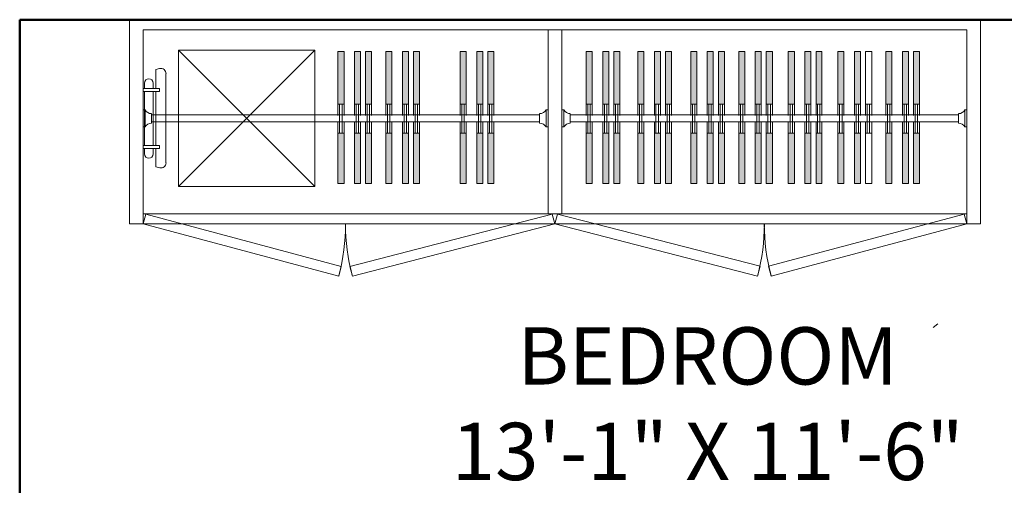
# Model space of a CAD drawing. Units: inches. Extents: x -466983 to 1020, y 324 to 318697.
# Tile 4 of 97: x 452 to 555, y 514 to 563. Entities that reach past the tile are written whole.
import ezdxf

# ---------------------------------------------------------------- set-up
doc = ezdxf.new("R2010")
doc.units = ezdxf.units.IN
doc.header["$MEASUREMENT"] = 0
for name, color, linetype, lineweight in [('A-AREA-IDEN', 7, 'Continuous', 25), ('A-FURN', 8, 'Continuous', 18), ('A-WALL', 7, 'Continuous', 50)]:
    doc.layers.add(name, color=color, linetype=linetype, lineweight=lineweight)
doc.styles.get("Standard").update_dxf_attribs({"font": 'arial.ttf'})

# ---------------------------------------------------------------- blocks, each defined once
blk = doc.blocks.new('A$C05F852CF')
for p, q in [((0.0306, 3.0783), (0.4692, 3.0783)), ((0.4692, 3.0783), (2.0768, 3.0783)), ((0.52, 3.0783), (0.52, 1.0783)), ((2.02, 3.0783), (2.02, 1.0783)), ((2.0768, 3.0783), (2.5066, 3.0783)), ((0, 3.0548), (0, 2.6659)), ((0.5, 3.0423), (0.5, 2.6496)), ((2.04, 3.05), (2.04, 2.6642)), ((0.52, 3.0283), (2.02, 3.0283)), ((2.54, 2.6547), (2.54, 3.0393)), ((0.2418, 2.9702), (0.2418, 3.0002)), ((0.5609, 3.0045), (0.5953, 2.9829)), ((0.5609, 3.0045), (0.6121, 2.9725)), ((1.2427, 2.9995), (1.1927, 2.9682)), ((2.2982, 2.9702), (2.2982, 3.0002)), ((0.6121, 2.9725), (0.6546, 2.9682)), ((1.1927, 2.9682), (1.1672, 2.9661)), ((0.1349, 2.8634), (0.1049, 2.8634)), ((0.3487, 2.8634), (0.3787, 2.8634)), ((2.1913, 2.8634), (2.1613, 2.8634)), ((2.4051, 2.8634), (2.4351, 2.8634)), ((0.2418, 2.7265), (0.2418, 2.7565)), ((2.2982, 2.7265), (2.2982, 2.7565)), ((0.5711, 2.6712), (0.6015, 2.7135)), ((0.6015, 2.7135), (0.6164, 2.7178)), ((1.1864, 2.7072), (1.1588, 2.7242)), ((1.2397, 2.6852), (1.1864, 2.7072)), ((1.0379, 2.6608), (0.52, 2.2697)), ((2.02, 2.6608), (1.0379, 2.6608)), ((1.7737, 2.6608), (1.7737, 1.0783)), ((1.7937, 2.6608), (1.7937, 1.0783)), ((1.8137, 2.6608), (1.8137, 1.0783)), ((1.8337, 2.6608), (1.8337, 1.0783)), ((0.0322, 2.6283), (0.4826, 2.6283)), ((2.0707, 2.6283), (2.5056, 2.6283)), ((0.52, 1.4597), (2.02, 1.4597)), ((0.52, 1.4397), (2.02, 1.4397)), ((0.52, 1.4197), (2.02, 1.4197)), ((0.52, 1.3997), (2.02, 1.3997)), ((0.52, 1.0783), (2.02, 1.0783)), ((0.726, 0.4346), (0.7377, 0.4444))]:
    blk.add_line(p, q)
for points in [[(1.3405, 2.9829), (1.306, 3.0045), (1.3573, 2.9725), (1.3998, 2.9682)], [(1.9879, 2.9995), (1.9379, 2.9682), (1.9124, 2.9661)], [(1.3162, 2.6712), (1.3467, 2.7135), (1.3616, 2.7178)], [(1.9848, 2.6852), (1.9315, 2.7072), (1.9039, 2.7242)]]:
    blk.add_lwpolyline(points)
for points in [[(1.0353, 2.1379, -0.173032), (1.022, 2.6388), (0.536, 2.2719, 0.053888)], [(1.7081, 1.7759, 0.101392), (1.7282, 1.7501, -0.223768), (1.7345, 1.736, -0.25558), (1.7315, 1.7308, -0.081563), (1.7151, 1.724, -0.071805), (1.6967, 1.7225, 0.069985), (1.6778, 1.7209, 0.03546), (1.6148, 1.7021, 0.029432), (1.5425, 1.6697, 0.001554), (1.5078, 1.6515, -0.00152), (1.4724, 1.6329, -0.004735), (1.4356, 1.6142, 0.00382), (1.3901, 1.5911, 0.296001), (1.3692, 1.5546, -0.649774), (1.3468, 1.5431, -0.02319), (1.3416, 1.5477, 0.0288), (1.3374, 1.5514, 0.005727), (1.3298, 1.557, -0.004358), (1.3198, 1.5645, -0.027528), (1.3001, 1.5812, -0.046214), (1.29, 1.5928, -0.194121), (1.2856, 1.6105, 0.133719), (1.2823, 1.6363, 0.011505), (1.2622, 1.682, 0.008882), (1.2338, 1.7401, 0.012426), (1.1937, 1.8139, -0.033612), (1.1801, 1.8418), (1.1552, 1.9026), (1.1361, 1.9495, 0.224341), (1.1204, 1.9638, -0.722772), (1.1202, 1.9734, -0.103513), (1.1242, 1.9739, 0.053465), (1.132, 1.9742, 0.030109), (1.1569, 1.9792, -0.031436), (1.1808, 1.984, -0.05324), (1.1971, 1.9844, 0.05518), (1.2128, 1.9849, 0.056271), (1.2402, 1.992, 0.0108), (1.3759, 2.0475, 0.00456), (1.4675, 2.0883, 0.01125), (1.5041, 2.106, 0.069394), (1.5235, 2.1196, -0.079756), (1.5405, 2.1311, -0.106399), (1.5562, 2.1345, -0.328642), (1.5608, 2.1312, -0.299547), (1.5587, 2.124, 0.189917), (1.5536, 2.1141, 0.033518), (1.5531, 2.1029, 0.075627), (1.554, 2.0981, 0.053489), (1.5579, 2.0898, 0.017838), (1.5727, 2.0672, 0.038394), (1.5932, 2.0425, -0.059529), (1.6058, 2.026, -0.035943), (1.6193, 1.9987, -0.011245), (1.6541, 1.9079, -0.006203), (1.6684, 1.8661, 0.010783), (1.6769, 1.8422, 0.019485), (1.6828, 1.8283, 0.005062)], [(1.6953, 1.7695, 0.098587), (1.7181, 1.7399, -0.040378), (1.7118, 1.7379, -0.071805), (1.6975, 1.7367, 0.069985), (1.6747, 1.7349, 0.03546), (1.6097, 1.7154, 0.029432), (1.5359, 1.6824, 0.001554), (1.5012, 1.6641, -0.00152), (1.4658, 1.6456, -0.004735), (1.4293, 1.627, 0.00382), (1.3835, 1.6038, 0.289814), (1.3549, 1.555, -0.018279), (1.3515, 1.5579, 0.0288), (1.3461, 1.5627, 0.005727), (1.3382, 1.5686, -0.004358), (1.3285, 1.5758, -0.027528), (1.31, 1.5916, -0.046214), (1.3016, 1.6012, -0.194121), (1.2997, 1.6085, 0.133719), (1.2955, 1.6417, 0.011505), (1.2752, 1.6881, 0.008882), (1.2465, 1.7466, 0.012426), (1.2061, 1.821, -0.033612), (1.1933, 1.8472), (1.1684, 1.908), (1.1493, 1.9549, 0.051417), (1.1455, 1.962, 0.017208), (1.1606, 1.9654, -0.031436), (1.1827, 1.9698, -0.05324), (1.196, 1.9702, 0.05518), (1.2149, 1.9708, 0.056271), (1.2453, 1.9787, 0.0108), (1.3816, 2.0344, 0.00456), (1.4734, 2.0753, 0.01125), (1.5106, 2.0933, 0.069394), (1.5332, 2.1091, -0.038161), (1.5392, 2.114, 0.029361), (1.5389, 2.1025, 0.075627), (1.5405, 2.0934, 0.053489), (1.5457, 2.0824, 0.017838), (1.5611, 2.0589, 0.038394), (1.583, 2.0326, -0.059529), (1.5935, 2.0187, -0.035943), (1.6061, 1.9933, -0.011245), (1.6406, 1.9031, -0.006203), (1.6549, 1.8617, 0.010783), (1.6635, 1.8371, 0.019485), (1.6699, 1.8222, 0.005062)]]:
    blk.add_lwpolyline(points, format="xyb", close=True)
for points in [[(1.27, 1.665, 0.025626), (1.2575, 1.662, 0.0108), (1.1179, 1.617, 0.00456), (1.0234, 1.5834, 0.01125), (0.9856, 1.5685, 0.069394), (0.9653, 1.5565, -0.079756), (0.9474, 1.5464, -0.106399), (0.9315, 1.5441, -0.328642), (0.9272, 1.5478, -0.299547), (0.9298, 1.5548, 0.189917), (0.9357, 1.5643, 0.033518), (0.9369, 1.5754, 0.075627), (0.9364, 1.5803, 0.053489), (0.9332, 1.5888, 0.017838), (0.9202, 1.6125, 0.038394), (0.9016, 1.6387, -0.059529), (0.8903, 1.6561, -0.035943), (0.8789, 1.6844, -0.011245), (0.8512, 1.7776, -0.006203), (0.8402, 1.8203, 0.010783), (0.8336, 1.8448, 0.019485), (0.8287, 1.8592, 0.005062), (0.8076, 1.9133, 0.101392), (0.7895, 1.9406, -0.223768), (0.7843, 1.9551, -0.25558), (0.7876, 1.9601, -0.081563), (0.8046, 1.9656, -0.071805), (0.823, 1.9657, 0.069985), (0.842, 1.9658, 0.03546), (0.9062, 1.9798, 0.029432), (0.9807, 2.0065, 0.001554), (1.0167, 2.022, -0.00152), (1.0535, 2.0378, -0.004735), (1.0916, 2.0536, 0.00382), (1.1388, 2.0731, 0.296001), (1.1624, 2.108, -0.649774), (1.1856, 2.1178, -0.02319), (1.1904, 2.1128, 0.0288), (1.1944, 2.1088, 0.005727), (1.2015, 2.1025, -0.004358), (1.2108, 2.0944, -0.027528), (1.2292, 2.0762, -0.046214), (1.2384, 2.0638, -0.194121), (1.2414, 2.0458, 0.133719), (1.2427, 2.0199, 0.005779), (1.2507, 1.9961)], [(1.2674, 1.6787, 0.025626), (1.2535, 1.6753, 0.0108), (1.1134, 1.6301, 0.00456), (1.0187, 1.5964, 0.01125), (0.9802, 1.5813, 0.069394), (0.9566, 1.5673, -0.042175), (0.9495, 1.5626, 0.031457), (0.9508, 1.5747, 0.075627), (0.9499, 1.5838, 0.053489), (0.9456, 1.595, 0.017838), (0.9321, 1.6196, 0.038394), (0.9123, 1.6476, -0.059529), (0.9028, 1.6622, -0.035943), (0.8922, 1.6886, -0.011245), (0.8646, 1.7812, -0.006203), (0.8536, 1.8236, 0.010783), (0.8469, 1.8487, 0.019485), (0.8417, 1.8641, 0.005062), (0.8204, 1.9185, 0.100237), (0.7996, 1.9501, -0.044209), (0.8066, 1.9519, -0.071805), (0.8211, 1.952, 0.069985), (0.8439, 1.9521, 0.03546), (0.9101, 1.9665, 0.029432), (0.9862, 1.9937, 0.001554), (1.0222, 2.0093, -0.00152), (1.0589, 2.025, -0.004735), (1.0968, 2.0408, 0.00382), (1.1442, 2.0604, 0.294287), (1.1763, 2.1074, -0.02184), (1.18, 2.1036, 0.0288), (1.1851, 2.0984, 0.005727), (1.1924, 2.092, -0.004358), (1.2016, 2.084, -0.027528), (1.2189, 2.0669, -0.046214), (1.2266, 2.0566, -0.194121), (1.2279, 2.0488, 0.133719), (1.2295, 2.0156, 0.005779), (1.2376, 1.9915, 0.005779)]]:
    blk.add_lwpolyline(points, format="xyb")
for centre, radius in [((0.2418, 2.8634), 0.1369), ((2.2982, 2.8634), 0.1369), ((0.2418, 2.8634), 0.1069), ((2.2982, 2.8634), 0.1069)]:
    blk.add_circle(centre, radius)
for centre, radius, start, end in [((1.7308, 2.407), 0.7379, 159.8846, 202.2194), ((1.4058, 4.5145), 2.4132, 248.4641, 261.4655)]:
    blk.add_arc(centre, radius, start, end)
for points in [[(0, 3.0548), (0, 3.0677), (0.0177, 3.0783), (0.0306, 3.0783)], [(0.5, 3.0423), (0.5, 3.0581), (0.485, 3.0783), (0.4692, 3.0783)], [(2.04, 3.05), (2.04, 3.0655), (2.0613, 3.0783), (2.0768, 3.0783)], [(2.5066, 3.0783), (2.5237, 3.0783), (2.54, 3.0564), (2.54, 3.0393)], [(0.0322, 2.6283), (0.0157, 2.6283), (0, 2.6494), (0, 2.6659)], [(2.04, 2.6642), (2.04, 2.6485), (2.055, 2.6283), (2.0707, 2.6283)], [(2.5056, 2.6283), (2.5201, 2.6283), (2.54, 2.6403), (2.54, 2.6547)], [(0.5, 2.6496), (0.5, 2.6405), (0.4918, 2.6283), (0.4826, 2.6283)]]:
    blk.add_open_spline(points, degree=3)
for points, knots in [([(0.5609, 3.0045), (0.565, 2.9818), (0.5836, 2.9366), (0.5776, 2.889), (0.5689, 2.8351), (0.5832, 2.7709), (0.5808, 2.7088), (0.5744, 2.6927), (0.5693, 2.6651), (0.5803, 2.6793), (0.5989, 2.6876), (0.7172, 2.6598), (0.8681, 2.7029), (1.0484, 2.6781), (1.0324, 2.6731), (1.1431, 2.7116), (1.202, 2.6757), (1.2459, 2.6867), (1.2222, 2.695), (1.2359, 2.7251), (1.2468, 2.781), (1.2288, 2.8492), (1.2515, 2.925), (1.2279, 2.9609), (1.2471, 3.0058), (1.2098, 2.9902), (1.1177, 3.0095), (0.956, 3.0159), (0.9532, 2.9758), (0.7999, 3.021), (0.7569, 3.0151), (0.5986, 2.9869), (0.561, 3.0049)], [16.816032, 16.816032, 16.816032, 16.816032, 79.038845, 88.513895, 147.565266, 227.196862, 259.685448, 283.955301, 296.511304, 302.432558, 320.230942, 354.322559, 575.279549, 734.72356, 845.740421, 943.033103, 1029.533967, 1032.845074, 1043.313584, 1065.311534, 1104.921835, 1208.53002, 1248.510714, 1303.102727, 1321.01326, 1329.647833, 1389.371624, 1571.817644, 1750.274161, 1823.189073, 1967.937033, 2020.912329, 2020.912329, 2020.912329, 2020.912329]), ([(1.306, 3.0045), (1.3102, 2.9818), (1.3287, 2.9366), (1.3228, 2.889), (1.314, 2.8351), (1.3284, 2.7709), (1.3259, 2.7088), (1.3196, 2.6927), (1.3144, 2.6651), (1.3254, 2.6793), (1.3441, 2.6876), (1.4624, 2.6598), (1.6132, 2.7029), (1.6436, 2.6781), (1.7775, 2.6731), (1.8882, 2.7116), (1.9472, 2.6757), (1.9911, 2.6867), (1.9673, 2.695), (1.981, 2.7251), (1.992, 2.781), (1.974, 2.8492), (1.9967, 2.925), (1.9731, 2.9609), (1.9922, 3.0058), (1.9549, 2.9902), (1.8628, 3.0095), (1.7011, 3.0159), (1.5483, 2.9758), (1.5451, 3.021), (1.5021, 3.0151), (1.3437, 2.9869), (1.3062, 3.0049)], [16.816032, 16.816032, 16.816032, 16.816032, 79.038845, 88.513895, 147.565266, 227.196862, 259.685448, 283.955301, 296.511304, 302.432558, 320.230942, 354.322559, 575.279549, 734.72356, 845.740421, 943.033103, 1029.533967, 1032.845074, 1043.313584, 1065.311534, 1104.921835, 1208.53002, 1248.510714, 1303.102727, 1321.01326, 1329.647833, 1389.371624, 1571.817644, 1750.274161, 1823.189073, 1967.937033, 2020.912329, 2020.912329, 2020.912329, 2020.912329]), ([(1.186, 2.943), (1.1557, 2.9456), (1.1387, 2.9502), (1.0976, 2.9551), (1.0776, 2.9567), (1.0342, 2.9582), (1.0123, 2.957), (0.991, 2.9533), (0.9902, 2.9517), (0.962, 2.9403), (0.9371, 2.935), (0.8851, 2.9413), (0.8522, 2.9513), (0.8033, 2.9629), (0.7938, 2.964), (0.755, 2.9608), (0.7319, 2.9572), (0.6794, 2.9481), (0.658, 2.9434), (0.631, 2.9418)], [1364.380335, 1364.380335, 1364.380335, 1364.380335, 1423.60231, 1423.60231, 1482.824284, 1482.824284, 1566.205036, 1566.205036, 1649.585789, 1649.585789, 1732.966542, 1732.966542, 1816.347295, 1816.347295, 1899.728048, 1899.728048, 1960.499853, 1960.499853, 1990.525565, 1990.525565, 1990.525565, 1990.525565]), ([(0.631, 2.9418), (0.6332, 2.9288), (0.633, 2.9104), (0.6308, 2.893), (0.6298, 2.8865), (0.628, 2.8726), (0.6273, 2.866), (0.6257, 2.8474), (0.6257, 2.8375), (0.629, 2.8013), (0.6345, 2.7696), (0.6337, 2.7333)], [67.285362, 67.285362, 67.285362, 67.285362, 87.399558, 87.399558, 107.513754, 107.513754, 127.62795, 127.62795, 167.856341, 167.856341, 238.127268, 238.127268, 238.127268, 238.127268]), ([(1.1845, 2.7412), (1.189, 2.7552), (1.1894, 2.765), (1.1874, 2.7998), (1.1843, 2.8219), (1.1844, 2.8664), (1.1882, 2.8901), (1.192, 2.9105), (1.1922, 2.9144), (1.1921, 2.9158), (1.1908, 2.9212), (1.1875, 2.9351), (1.1867, 2.9388), (1.186, 2.943)], [1072.516901, 1072.516901, 1072.516901, 1072.516901, 1129.100964, 1129.100964, 1185.685027, 1185.685027, 1226.035089, 1226.035089, 1249.281274, 1249.281274, 1272.52746, 1272.52746, 1279.689275, 1279.689275, 1279.689275, 1279.689275]), ([(1.3759, 2.942), (1.3781, 2.929), (1.378, 2.9106), (1.3757, 2.893), (1.3748, 2.8866), (1.373, 2.8727), (1.3722, 2.8661), (1.3706, 2.8475), (1.3707, 2.8375), (1.3739, 2.8012), (1.3795, 2.7694), (1.3787, 2.7331)], [67.156228, 67.156228, 67.156228, 67.156228, 87.297212, 87.297212, 107.438196, 107.438196, 127.57918, 127.57918, 167.861148, 167.861148, 238.25357, 238.25357, 238.25357, 238.25357]), ([(1.5104, 2.9621), (1.4964, 2.9606), (1.4732, 2.9568), (1.4226, 2.948), (1.4017, 2.9435), (1.3759, 2.942)], [1904.3965, 1904.3965, 1904.3965, 1904.3965, 1961.927876, 1961.927876, 1990.619445, 1990.619445, 1990.619445, 1990.619445]), ([(1.9314, 2.9432), (1.8997, 2.9459), (1.8822, 2.9507), (1.8387, 2.9557), (1.8168, 2.9572), (1.7515, 2.9587), (1.7088, 2.9551), (1.6403, 2.9447), (1.6154, 2.9402), (1.5795, 2.937), (1.5675, 2.9361), (1.5394, 2.9412), (1.5201, 2.9507), (1.5104, 2.9621)], [1364.265661, 1364.265661, 1364.265661, 1364.265661, 1426.240795, 1426.240795, 1488.215928, 1488.215928, 1612.166195, 1612.166195, 1689.92864, 1689.92864, 1733.064362, 1733.064362, 1768.978829, 1768.978829, 1768.978829, 1768.978829]), ([(1.9299, 2.7409), (1.9344, 2.755), (1.9348, 2.7648), (1.9328, 2.7996), (1.9297, 2.8217), (1.9298, 2.8662), (1.9336, 2.8899), (1.9374, 2.9105), (1.9376, 2.9144), (1.9375, 2.9159), (1.9362, 2.9214), (1.9329, 2.9353), (1.9321, 2.939), (1.9314, 2.9432)], [1072.238498, 1072.238498, 1072.238498, 1072.238498, 1128.864869, 1128.864869, 1185.491239, 1185.491239, 1225.989553, 1225.989553, 1249.326401, 1249.326401, 1272.66325, 1272.66325, 1279.788508, 1279.788508, 1279.788508, 1279.788508]), ([(0.6337, 2.7333), (0.6515, 2.7301), (0.6627, 2.7284), (0.6898, 2.7263), (0.7032, 2.726), (0.7436, 2.727), (0.7707, 2.73), (0.8409, 2.7383), (0.8881, 2.7432), (0.9755, 2.7406), (1.0125, 2.7357), (1.0356, 2.7309), (1.0369, 2.7307), (1.0381, 2.7304)], [345.4047, 345.4047, 345.4047, 345.4047, 383.386056, 383.386056, 421.367413, 421.367413, 497.330126, 497.330126, 611.561469, 611.561469, 725.792813, 725.792813, 732.434768, 732.434768, 732.434768, 732.434768]), ([(1.0381, 2.7304), (1.0497, 2.7345), (1.0742, 2.7435), (1.1251, 2.7504), (1.1528, 2.749), (1.1769, 2.7432), (1.1809, 2.7421), (1.1845, 2.7412)], [843.64503, 843.64503, 843.64503, 843.64503, 911.27572, 911.27572, 959.088062, 959.088062, 969.47998, 969.47998, 969.47998, 969.47998]), ([(1.3787, 2.7331), (1.3984, 2.7296), (1.4106, 2.7278), (1.4401, 2.7258), (1.4545, 2.7258), (1.4962, 2.7276), (1.5219, 2.7313), (1.5767, 2.7399), (1.6067, 2.7436), (1.6527, 2.7371), (1.662, 2.7326), (1.7084, 2.7282), (1.7364, 2.7276), (1.7849, 2.734), (1.8076, 2.7406), (1.8563, 2.7489), (1.8812, 2.7508), (1.914, 2.7451), (1.9226, 2.7428), (1.9299, 2.7409)], [345.267918, 345.267918, 345.267918, 345.267918, 387.167414, 387.167414, 429.06691, 429.06691, 512.865903, 512.865903, 629.317545, 629.317545, 745.769188, 745.769188, 834.622813, 834.622813, 901.414409, 901.414409, 948.921878, 948.921878, 969.679511, 969.679511, 969.679511, 969.679511])]:
    blk.add_open_spline(points, degree=3, knots=knots)
for p in [(0.2366, 2.8475), (2.3034, 2.8475), (0.2309, 2.8244), (2.02, 1.0783), (2.02, 1.0783)]:
    blk.add_point(p)
blk = doc.blocks.new('Wardrobe')
h = blk.add_hatch(color=256)
h.dxf.hatch_style = 1
h.paths.add_polyline_path([(2766.95, 1539.75), (2766.16, 1539.75), (2766.16, 1532.86), (2766.95, 1532.86)])
h.paths.add_polyline_path([(2766.95, 1529.07), (2766.16, 1529.07), (2766.16, 1522.48), (2766.95, 1522.48)])
h.paths.add_polyline_path([(2799.41, 1529.07), (2798.63, 1529.07), (2798.63, 1522.47), (2799.41, 1522.47)])
h.paths.add_polyline_path([(2799.41, 1539.75), (2798.63, 1539.75), (2798.63, 1532.86), (2799.41, 1532.86)])
h.paths.add_polyline_path([(2813.08, 1539.75), (2812.29, 1539.75), (2812.29, 1532.86), (2813.08, 1532.86)])
h.paths.add_polyline_path([(2813.08, 1529.07), (2812.29, 1529.07), (2812.29, 1522.47), (2813.08, 1522.47)])
h.paths.add_polyline_path([(2825.84, 1539.75), (2825.05, 1539.75), (2825.05, 1532.86), (2825.84, 1532.86)])
h.paths.add_polyline_path([(2825.84, 1529.07), (2825.05, 1529.07), (2825.05, 1522.47), (2825.84, 1522.47)])
h.paths.add_polyline_path([(2782.93, 1539.75), (2782.14, 1539.75), (2782.14, 1532.86), (2782.93, 1532.86)])
h.paths.add_polyline_path([(2782.93, 1529.07), (2782.14, 1529.07), (2782.14, 1522.48), (2782.93, 1522.48)])
h.paths.add_polyline_path([(2838.6, 1539.75), (2837.81, 1539.75), (2837.81, 1532.86), (2838.6, 1532.86)])
h.paths.add_polyline_path([(2838.6, 1529.07), (2837.81, 1529.07), (2837.81, 1522.47), (2838.6, 1522.47)])
h = blk.add_hatch(color=256)
h.dxf.hatch_style = 1
h.paths.add_polyline_path([(2769.11, 1539.75), (2768.32, 1539.75), (2768.32, 1532.86), (2769.11, 1532.86)])
h.paths.add_polyline_path([(2769.11, 1529.07), (2768.32, 1529.07), (2768.32, 1522.48), (2769.11, 1522.48)])
h.paths.add_polyline_path([(2801.57, 1539.75), (2800.79, 1539.75), (2800.79, 1532.86), (2801.57, 1532.86)])
h.paths.add_polyline_path([(2801.57, 1529.07), (2800.79, 1529.07), (2800.79, 1522.47), (2801.57, 1522.47)])
h.paths.add_polyline_path([(2815.24, 1539.75), (2814.45, 1539.75), (2814.45, 1532.86), (2815.24, 1532.86)])
h.paths.add_polyline_path([(2815.24, 1529.07), (2814.45, 1529.07), (2814.45, 1522.47), (2815.24, 1522.47)])
h.paths.add_polyline_path([(2828, 1529.07), (2827.21, 1529.07), (2827.21, 1522.47), (2828, 1522.47)])
h.paths.add_polyline_path([(2828, 1539.75), (2827.21, 1539.75), (2827.21, 1532.86), (2828, 1532.86)])
h.paths.add_polyline_path([(2840.76, 1539.75), (2839.97, 1539.75), (2839.97, 1532.86), (2840.76, 1532.86)])
h.paths.add_polyline_path([(2840.76, 1529.07), (2839.97, 1529.07), (2839.97, 1522.47), (2840.76, 1522.47)])
h.paths.add_polyline_path([(2785.09, 1539.75), (2784.3, 1539.75), (2784.3, 1532.86), (2785.09, 1532.86)])
h.paths.add_polyline_path([(2785.09, 1529.07), (2784.3, 1529.07), (2784.3, 1522.48), (2785.09, 1522.48)])
h = blk.add_hatch(color=256)
h.dxf.hatch_style = 1
h.paths.add_polyline_path([(2770.56, 1539.75), (2769.77, 1539.75), (2769.77, 1532.86), (2770.56, 1532.86)])
h.paths.add_polyline_path([(2770.56, 1529.07), (2769.77, 1529.07), (2769.77, 1522.48), (2770.56, 1522.48)])
h.paths.add_polyline_path([(2786.54, 1539.75), (2785.76, 1539.75), (2785.76, 1532.86), (2786.54, 1532.86)])
h.paths.add_polyline_path([(2786.54, 1529.07), (2785.76, 1529.07), (2785.76, 1522.48), (2786.54, 1522.48)])
h.paths.add_polyline_path([(2803.03, 1539.75), (2802.24, 1539.75), (2802.24, 1532.86), (2803.03, 1532.86)])
h.paths.add_polyline_path([(2803.03, 1529.07), (2802.24, 1529.07), (2802.24, 1522.47), (2803.03, 1522.47)])
h.paths.add_polyline_path([(2816.69, 1539.75), (2815.9, 1539.75), (2815.9, 1532.86), (2816.69, 1532.86)])
h.paths.add_polyline_path([(2816.69, 1529.07), (2815.9, 1529.07), (2815.9, 1522.47), (2816.69, 1522.47)])
h = blk.add_hatch(color=256)
h.dxf.hatch_style = 1
h.paths.add_polyline_path([(2773.22, 1539.75), (2772.43, 1539.75), (2772.43, 1532.86), (2773.22, 1532.86)])
h.paths.add_polyline_path([(2806.16, 1539.75), (2805.37, 1539.75), (2805.37, 1532.86), (2806.16, 1532.86)])
h.paths.add_polyline_path([(2806.16, 1529.07), (2805.37, 1529.07), (2805.37, 1522.47), (2806.16, 1522.47)])
h.paths.add_polyline_path([(2773.22, 1529.07), (2772.43, 1529.07), (2772.43, 1522.48), (2773.22, 1522.48)])
h.paths.add_polyline_path([(2819.35, 1539.75), (2818.56, 1539.75), (2818.56, 1532.86), (2819.35, 1532.86)])
h.paths.add_polyline_path([(2819.35, 1529.07), (2818.56, 1529.07), (2818.56, 1522.47), (2819.35, 1522.47)])
h.paths.add_polyline_path([(2832.33, 1539.75), (2831.54, 1539.75), (2831.54, 1532.86), (2832.33, 1532.86)])
h.paths.add_polyline_path([(2832.33, 1529.07), (2831.54, 1529.07), (2831.54, 1522.47), (2832.33, 1522.47)])
h = blk.add_hatch(color=256)
h.dxf.hatch_style = 1
h.paths.add_polyline_path([(2775.38, 1539.75), (2774.59, 1539.75), (2774.59, 1532.86), (2775.38, 1532.86)])
h.paths.add_polyline_path([(2775.38, 1529.07), (2774.59, 1529.07), (2774.59, 1522.48), (2775.38, 1522.48)])
h.paths.add_polyline_path([(2808.32, 1539.75), (2807.53, 1539.75), (2807.53, 1532.86), (2808.32, 1532.86)])
h.paths.add_polyline_path([(2808.32, 1529.07), (2807.53, 1529.07), (2807.53, 1522.47), (2808.32, 1522.47)])
h.paths.add_polyline_path([(2834.49, 1539.75), (2833.7, 1539.75), (2833.7, 1532.86), (2834.49, 1532.86)])
h.paths.add_polyline_path([(2834.49, 1529.07), (2833.7, 1529.07), (2833.7, 1522.47), (2834.49, 1522.47)])
h = blk.add_hatch(color=256)
h.dxf.hatch_style = 1
h.paths.add_polyline_path([(2776.83, 1539.75), (2776.04, 1539.75), (2776.04, 1532.86), (2776.83, 1532.86)])
h.paths.add_polyline_path([(2776.83, 1529.07), (2776.04, 1529.07), (2776.04, 1522.48), (2776.83, 1522.48)])
h.paths.add_polyline_path([(2809.77, 1539.75), (2808.98, 1539.75), (2808.98, 1532.86), (2809.77, 1532.86)])
h.paths.add_polyline_path([(2809.77, 1529.07), (2808.98, 1529.07), (2808.98, 1522.47), (2809.77, 1522.47)])
h.paths.add_polyline_path([(2821.51, 1539.75), (2820.72, 1539.75), (2820.72, 1532.86), (2821.51, 1532.86)])
h.paths.add_polyline_path([(2821.51, 1529.07), (2820.72, 1529.07), (2820.72, 1522.47), (2821.51, 1522.47)])
h = blk.add_hatch(color=256)
h.dxf.hatch_style = 1
h.paths.add_polyline_path([(2822.96, 1539.75), (2822.17, 1539.75), (2822.17, 1532.86), (2822.96, 1532.86)])
h.paths.add_polyline_path([(2822.96, 1529.07), (2822.17, 1529.07), (2822.17, 1522.47), (2822.96, 1522.47)])
h = blk.add_hatch(color=256)
h.dxf.hatch_style = 1
h.paths.add_polyline_path([(2829.45, 1539.75), (2828.67, 1539.75), (2828.67, 1532.86), (2829.45, 1532.86)])
h.paths.add_polyline_path([(2829.45, 1529.07), (2828.67, 1529.07), (2828.67, 1522.47), (2829.45, 1522.47)])
h.paths.add_polyline_path([(2842.22, 1539.75), (2841.43, 1539.75), (2841.43, 1532.86), (2842.22, 1532.86)])
h.paths.add_polyline_path([(2842.22, 1529.07), (2841.43, 1529.07), (2841.43, 1522.47), (2842.22, 1522.47)])
for p, q in [((2738.89, 1517.19, 0), (2738.89, 1543.9, 0)), ((2738.89, 1543.9, 0), (2850.18, 1543.9, 0)), ((2850.18, 1543.9, 0), (2850.18, 1517.19, 0)), ((2848.4, 1542.57, 0), (2740.67, 1542.57, 0)), ((2740.67, 1542.57, 0), (2740.67, 1517.19, 0)), ((2793.64, 1542.57, 0), (2793.64, 1518.53, 0)), ((2795.43, 1542.57, 0), (2795.43, 1518.53, 0)), ((2848.4, 1517.19, 0), (2848.4, 1542.57, 0)), ((2740.94, 1532.1, 0), (2740.67, 1532.1, 0)), ((2740.94, 1532.1, 0), (2740.67, 1532.1, 0)), ((2740.94, 1532.1, 0), (2740.94, 1529.88, 0)), ((2740.94, 1532.1, 0), (2740.94, 1529.88, 0)), ((2741.78, 1531.61, 0), (2741.78, 1530.37, 0)), ((2741.78, 1531.45, 0), (2792.53, 1531.45, 0)), ((2792.53, 1531.61, 0), (2792.53, 1530.37, 0)), ((2793.38, 1532.1, 0), (2793.38, 1529.88, 0)), ((2793.38, 1532.1, 0), (2793.38, 1529.88, 0)), ((2793.38, 1532.1, 0), (2793.64, 1532.1, 0)), ((2793.38, 1532.1, 0), (2793.64, 1532.1, 0)), ((2795.69, 1532.1, 0), (2795.43, 1532.1, 0)), ((2795.69, 1532.1, 0), (2795.43, 1532.1, 0)), ((2795.69, 1532.1, 0), (2795.69, 1529.88, 0)), ((2795.69, 1532.1, 0), (2795.69, 1529.88, 0)), ((2796.54, 1531.61, 0), (2796.54, 1530.37, 0)), ((2796.54, 1531.45, 0), (2847.29, 1531.45, 0)), ((2847.29, 1531.61, 0), (2847.29, 1530.37, 0)), ((2848.13, 1532.1, 0), (2848.13, 1529.88, 0)), ((2848.13, 1532.1, 0), (2848.13, 1529.88, 0)), ((2848.13, 1532.1, 0), (2848.4, 1532.1, 0)), ((2848.13, 1532.1, 0), (2848.4, 1532.1, 0)), ((2740.94, 1529.88, 0), (2740.67, 1529.88, 0)), ((2740.94, 1529.88, 0), (2740.67, 1529.88, 0)), ((2741.78, 1530.56, 0), (2792.53, 1530.56, 0)), ((2793.38, 1529.88, 0), (2793.64, 1529.88, 0)), ((2793.38, 1529.88, 0), (2793.64, 1529.88, 0)), ((2795.69, 1529.88, 0), (2795.43, 1529.88, 0)), ((2795.69, 1529.88, 0), (2795.43, 1529.88, 0)), ((2796.54, 1530.56, 0), (2847.29, 1530.56, 0)), ((2848.13, 1529.88, 0), (2848.4, 1529.88, 0)), ((2848.13, 1529.88, 0), (2848.4, 1529.88, 0)), ((2848.4, 1518.53, 0), (2740.67, 1518.53, 0)), ((2740.67, 1517.19, 0), (2741.02, 1518.48, 0)), ((2741.02, 1518.48, 0), (2766.6, 1511.65, 0)), ((2794.19, 1518.48, 0), (2767.71, 1511.65, 0)), ((2795.43, 1518.53, 0), (2793.64, 1518.53, 0)), ((2794.53, 1517.19, 0), (2794.19, 1518.48, 0)), ((2794.53, 1517.19, 0), (2794.88, 1518.48, 0)), ((2794.88, 1518.48, 0), (2821.36, 1511.66, 0)), ((2848.05, 1518.48, 0), (2822.47, 1511.66, 0)), ((2848.4, 1517.19, 0), (2848.05, 1518.48, 0)), ((2740.67, 1517.19, 0), (2738.89, 1517.19, 0)), ((2848.4, 1517.19, 0), (2740.67, 1517.19, 0)), ((2766.26, 1510.37, 0), (2740.67, 1517.19, 0)), ((2768.06, 1510.37, 0), (2794.53, 1517.19, 0)), ((2821.01, 1510.37, 0), (2794.53, 1517.19, 0)), ((2822.81, 1510.37, 0), (2848.4, 1517.19, 0)), ((2850.18, 1517.19, 0), (2848.4, 1517.19, 0)), ((2766.6, 1511.65, 0), (2766.26, 1510.37, 0)), ((2767.71, 1511.65, 0), (2768.06, 1510.37, 0)), ((2821.36, 1511.66, 0), (2821.01, 1510.37, 0)), ((2822.47, 1511.66, 0), (2822.81, 1510.37, 0))]:
    blk.add_line(p, q)
at = {"ltscale": 0.106667}
for p, q in [((2745.32, 1522.09, 0), (2763.13, 1539.9, 0)), ((2745.32, 1522.09, 0), (2745.32, 1539.9, 0)), ((2745.32, 1539.9, 0), (2763.13, 1539.9, 0)), ((2763.13, 1522.09, 0), (2745.32, 1539.9, 0)), ((2763.13, 1539.9, 0), (2763.13, 1522.09, 0)), ((2763.13, 1522.09, 0), (2745.32, 1522.09, 0))]:
    blk.add_line(p, q, dxfattribs=at)
at = {"ltscale": 0.037333}
for p, q in [((2766.16, 1531.37, 0), (2766.16, 1539.75, 0)), ((2766.16, 1539.75, 0), (2766.95, 1539.75, 0)), ((2766.95, 1539.75, 0), (2766.95, 1531.37, 0)), ((2768.32, 1531.37, 0), (2768.32, 1539.75, 0)), ((2768.32, 1539.75, 0), (2769.11, 1539.75, 0)), ((2769.11, 1539.75, 0), (2769.11, 1531.37, 0)), ((2769.77, 1531.37, 0), (2769.77, 1539.75, 0)), ((2769.77, 1539.75, 0), (2770.56, 1539.75, 0)), ((2770.56, 1539.75, 0), (2770.56, 1531.37, 0)), ((2772.43, 1531.37, 0), (2772.43, 1539.75, 0)), ((2772.43, 1539.75, 0), (2773.22, 1539.75, 0)), ((2773.22, 1539.75, 0), (2773.22, 1531.37, 0)), ((2774.59, 1531.37, 0), (2774.59, 1539.75, 0)), ((2774.59, 1539.75, 0), (2775.38, 1539.75, 0)), ((2775.38, 1539.75, 0), (2775.38, 1531.37, 0)), ((2776.04, 1531.37, 0), (2776.04, 1539.75, 0)), ((2776.04, 1539.75, 0), (2776.83, 1539.75, 0)), ((2776.83, 1539.75, 0), (2776.83, 1531.37, 0)), ((2782.14, 1531.37, 0), (2782.14, 1539.75, 0)), ((2782.14, 1539.75, 0), (2782.93, 1539.75, 0)), ((2782.93, 1539.75, 0), (2782.93, 1531.37, 0)), ((2784.3, 1531.37, 0), (2784.3, 1539.75, 0)), ((2784.3, 1539.75, 0), (2785.09, 1539.75, 0)), ((2785.09, 1539.75, 0), (2785.09, 1531.37, 0)), ((2785.76, 1531.37, 0), (2785.76, 1539.75, 0)), ((2785.76, 1539.75, 0), (2786.54, 1539.75, 0)), ((2786.54, 1539.75, 0), (2786.54, 1531.37, 0)), ((2798.63, 1531.36, 0), (2798.63, 1539.75, 0)), ((2798.63, 1539.75, 0), (2799.41, 1539.75, 0)), ((2799.41, 1539.75, 0), (2799.41, 1531.36, 0)), ((2800.79, 1531.36, 0), (2800.79, 1539.75, 0)), ((2800.79, 1539.75, 0), (2801.57, 1539.75, 0)), ((2801.57, 1539.75, 0), (2801.57, 1531.36, 0)), ((2802.24, 1531.36, 0), (2802.24, 1539.75, 0)), ((2802.24, 1539.75, 0), (2803.03, 1539.75, 0)), ((2803.03, 1539.75, 0), (2803.03, 1531.36, 0)), ((2805.37, 1531.36, 0), (2805.37, 1539.75, 0)), ((2805.37, 1539.75, 0), (2806.16, 1539.75, 0)), ((2806.16, 1539.75, 0), (2806.16, 1531.36, 0)), ((2807.53, 1531.36, 0), (2807.53, 1539.75, 0)), ((2807.53, 1539.75, 0), (2808.32, 1539.75, 0)), ((2808.32, 1539.75, 0), (2808.32, 1531.36, 0)), ((2808.98, 1531.36, 0), (2808.98, 1539.75, 0)), ((2808.98, 1539.75, 0), (2809.77, 1539.75, 0)), ((2809.77, 1539.75, 0), (2809.77, 1531.36, 0)), ((2812.29, 1531.36, 0), (2812.29, 1539.75, 0)), ((2812.29, 1539.75, 0), (2813.08, 1539.75, 0)), ((2813.08, 1539.75, 0), (2813.08, 1531.36, 0)), ((2814.45, 1531.36, 0), (2814.45, 1539.75, 0)), ((2814.45, 1539.75, 0), (2815.24, 1539.75, 0)), ((2815.24, 1539.75, 0), (2815.24, 1531.36, 0)), ((2815.9, 1531.36, 0), (2815.9, 1539.75, 0)), ((2815.9, 1539.75, 0), (2816.69, 1539.75, 0)), ((2816.69, 1539.75, 0), (2816.69, 1531.36, 0)), ((2818.56, 1531.36, 0), (2818.56, 1539.75, 0)), ((2818.56, 1539.75, 0), (2819.35, 1539.75, 0)), ((2819.35, 1539.75, 0), (2819.35, 1531.36, 0)), ((2820.72, 1531.36, 0), (2820.72, 1539.75, 0)), ((2820.72, 1539.75, 0), (2821.51, 1539.75, 0)), ((2821.51, 1539.75, 0), (2821.51, 1531.36, 0)), ((2822.17, 1531.36, 0), (2822.17, 1539.75, 0)), ((2822.17, 1539.75, 0), (2822.96, 1539.75, 0)), ((2822.96, 1539.75, 0), (2822.96, 1531.36, 0)), ((2825.05, 1531.36, 0), (2825.05, 1539.75, 0)), ((2825.05, 1539.75, 0), (2825.84, 1539.75, 0)), ((2825.84, 1539.75, 0), (2825.84, 1531.36, 0)), ((2827.21, 1531.36, 0), (2827.21, 1539.75, 0)), ((2827.21, 1539.75, 0), (2828, 1539.75, 0)), ((2828, 1539.75, 0), (2828, 1531.36, 0)), ((2828.67, 1531.36, 0), (2828.67, 1539.75, 0)), ((2828.67, 1539.75, 0), (2829.45, 1539.75, 0)), ((2829.45, 1539.75, 0), (2829.45, 1531.36, 0)), ((2831.54, 1531.36, 0), (2831.54, 1539.75, 0)), ((2831.54, 1539.75, 0), (2832.33, 1539.75, 0)), ((2832.33, 1539.75, 0), (2832.33, 1531.36, 0)), ((2833.7, 1531.36, 0), (2833.7, 1539.75, 0)), ((2833.7, 1539.75, 0), (2834.49, 1539.75, 0)), ((2834.49, 1539.75, 0), (2834.49, 1531.36, 0)), ((2835.16, 1531.36, 0), (2835.16, 1539.75, 0)), ((2835.16, 1539.75, 0), (2835.95, 1539.75, 0)), ((2835.95, 1539.75, 0), (2835.95, 1531.36, 0)), ((2837.81, 1531.36, 0), (2837.81, 1539.75, 0)), ((2837.81, 1539.75, 0), (2838.6, 1539.75, 0)), ((2838.6, 1539.75, 0), (2838.6, 1531.36, 0)), ((2839.97, 1531.36, 0), (2839.97, 1539.75, 0)), ((2839.97, 1539.75, 0), (2840.76, 1539.75, 0)), ((2840.76, 1539.75, 0), (2840.76, 1531.36, 0)), ((2841.43, 1531.36, 0), (2841.43, 1539.75, 0)), ((2841.43, 1539.75, 0), (2842.22, 1539.75, 0)), ((2842.22, 1539.75, 0), (2842.22, 1531.36, 0)), ((2766.16, 1532.86, 0), (2766.95, 1532.86, 0)), ((2766.37, 1529.07, 0), (2766.37, 1532.86, 0)), ((2766.69, 1529.07, 0), (2766.69, 1532.86, 0)), ((2768.32, 1532.86, 0), (2769.11, 1532.86, 0)), ((2768.53, 1529.07, 0), (2768.53, 1532.86, 0)), ((2768.84, 1529.07, 0), (2768.84, 1532.86, 0)), ((2769.77, 1532.86, 0), (2770.56, 1532.86, 0)), ((2769.99, 1529.07, 0), (2769.99, 1532.86, 0)), ((2770.3, 1529.07, 0), (2770.3, 1532.86, 0)), ((2772.43, 1532.86, 0), (2773.22, 1532.86, 0)), ((2772.64, 1529.07, 0), (2772.64, 1532.86, 0)), ((2772.96, 1529.07, 0), (2772.96, 1532.86, 0)), ((2774.59, 1532.86, 0), (2775.38, 1532.86, 0)), ((2774.8, 1529.07, 0), (2774.8, 1532.86, 0)), ((2775.11, 1529.07, 0), (2775.11, 1532.86, 0)), ((2776.04, 1532.86, 0), (2776.83, 1532.86, 0)), ((2776.26, 1529.07, 0), (2776.26, 1532.86, 0)), ((2776.57, 1529.07, 0), (2776.57, 1532.86, 0)), ((2782.14, 1532.86, 0), (2782.93, 1532.86, 0)), ((2782.36, 1529.07, 0), (2782.36, 1532.86, 0)), ((2782.67, 1529.07, 0), (2782.67, 1532.86, 0)), ((2784.3, 1532.86, 0), (2785.09, 1532.86, 0)), ((2784.52, 1529.07, 0), (2784.52, 1532.86, 0)), ((2784.83, 1529.07, 0), (2784.83, 1532.86, 0)), ((2785.76, 1532.86, 0), (2786.54, 1532.86, 0)), ((2785.97, 1529.07, 0), (2785.97, 1532.86, 0)), ((2786.28, 1529.07, 0), (2786.28, 1532.86, 0)), ((2798.63, 1532.86, 0), (2799.41, 1532.86, 0)), ((2798.84, 1529.07, 0), (2798.84, 1532.86, 0)), ((2799.15, 1529.07, 0), (2799.15, 1532.86, 0)), ((2800.79, 1532.86, 0), (2801.57, 1532.86, 0)), ((2801, 1529.07, 0), (2801, 1532.86, 0)), ((2801.31, 1529.07, 0), (2801.31, 1532.86, 0)), ((2802.24, 1532.86, 0), (2803.03, 1532.86, 0)), ((2802.45, 1529.07, 0), (2802.45, 1532.86, 0)), ((2802.76, 1529.07, 0), (2802.76, 1532.86, 0)), ((2805.37, 1532.86, 0), (2806.16, 1532.86, 0)), ((2805.58, 1529.07, 0), (2805.58, 1532.86, 0)), ((2805.9, 1529.07, 0), (2805.9, 1532.86, 0)), ((2807.53, 1532.86, 0), (2808.32, 1532.86, 0)), ((2807.74, 1529.07, 0), (2807.74, 1532.86, 0)), ((2808.06, 1529.07, 0), (2808.06, 1532.86, 0)), ((2808.98, 1532.86, 0), (2809.77, 1532.86, 0)), ((2809.2, 1529.07, 0), (2809.2, 1532.86, 0)), ((2809.51, 1529.07, 0), (2809.51, 1532.86, 0)), ((2812.29, 1532.86, 0), (2813.08, 1532.86, 0)), ((2812.51, 1529.07, 0), (2812.51, 1532.86, 0)), ((2812.82, 1529.07, 0), (2812.82, 1532.86, 0)), ((2814.45, 1532.86, 0), (2815.24, 1532.86, 0)), ((2814.67, 1529.07, 0), (2814.67, 1532.86, 0)), ((2814.98, 1529.07, 0), (2814.98, 1532.86, 0)), ((2815.9, 1532.86, 0), (2816.69, 1532.86, 0)), ((2816.12, 1529.07, 0), (2816.12, 1532.86, 0)), ((2816.43, 1529.07, 0), (2816.43, 1532.86, 0)), ((2818.56, 1532.86, 0), (2819.35, 1532.86, 0)), ((2818.78, 1529.07, 0), (2818.78, 1532.86, 0)), ((2819.09, 1529.07, 0), (2819.09, 1532.86, 0)), ((2820.72, 1532.86, 0), (2821.51, 1532.86, 0)), ((2820.94, 1529.07, 0), (2820.94, 1532.86, 0)), ((2821.25, 1529.07, 0), (2821.25, 1532.86, 0)), ((2822.17, 1532.86, 0), (2822.96, 1532.86, 0)), ((2822.39, 1529.07, 0), (2822.39, 1532.86, 0)), ((2822.7, 1529.07, 0), (2822.7, 1532.86, 0)), ((2825.05, 1532.86, 0), (2825.84, 1532.86, 0)), ((2825.27, 1529.07, 0), (2825.27, 1532.86, 0)), ((2825.58, 1529.07, 0), (2825.58, 1532.86, 0)), ((2827.21, 1532.86, 0), (2828, 1532.86, 0)), ((2827.43, 1529.07, 0), (2827.43, 1532.86, 0)), ((2827.74, 1529.07, 0), (2827.74, 1532.86, 0)), ((2828.67, 1532.86, 0), (2829.45, 1532.86, 0)), ((2828.88, 1529.07, 0), (2828.88, 1532.86, 0)), ((2829.19, 1529.07, 0), (2829.19, 1532.86, 0)), ((2831.54, 1532.86, 0), (2832.33, 1532.86, 0)), ((2831.76, 1529.07, 0), (2831.76, 1532.86, 0)), ((2832.07, 1529.07, 0), (2832.07, 1532.86, 0)), ((2833.7, 1532.86, 0), (2834.49, 1532.86, 0)), ((2833.92, 1529.07, 0), (2833.92, 1532.86, 0)), ((2834.23, 1529.07, 0), (2834.23, 1532.86, 0)), ((2835.16, 1532.86, 0), (2835.95, 1532.86, 0)), ((2835.37, 1529.07, 0), (2835.37, 1532.86, 0)), ((2835.68, 1529.07, 0), (2835.68, 1532.86, 0)), ((2837.81, 1532.86, 0), (2838.6, 1532.86, 0)), ((2838.03, 1529.07, 0), (2838.03, 1532.86, 0)), ((2838.34, 1529.07, 0), (2838.34, 1532.86, 0)), ((2839.97, 1532.86, 0), (2840.76, 1532.86, 0)), ((2840.19, 1529.07, 0), (2840.19, 1532.86, 0)), ((2840.5, 1529.07, 0), (2840.5, 1532.86, 0)), ((2841.43, 1532.86, 0), (2842.22, 1532.86, 0)), ((2841.64, 1529.07, 0), (2841.64, 1532.86, 0)), ((2841.95, 1529.07, 0), (2841.95, 1532.86, 0)), ((2766.16, 1522.48, 0), (2766.16, 1530.56, 0)), ((2766.95, 1530.56, 0), (2766.95, 1522.48, 0)), ((2768.32, 1522.48, 0), (2768.32, 1530.56, 0)), ((2769.11, 1530.56, 0), (2769.11, 1522.48, 0)), ((2769.77, 1522.48, 0), (2769.77, 1530.56, 0)), ((2770.56, 1530.56, 0), (2770.56, 1522.48, 0)), ((2772.43, 1522.48, 0), (2772.43, 1530.56, 0)), ((2773.22, 1530.56, 0), (2773.22, 1522.48, 0)), ((2774.59, 1522.48, 0), (2774.59, 1530.56, 0)), ((2775.38, 1530.56, 0), (2775.38, 1522.48, 0)), ((2776.04, 1522.48, 0), (2776.04, 1530.56, 0)), ((2776.83, 1530.56, 0), (2776.83, 1522.48, 0)), ((2782.14, 1522.48, 0), (2782.14, 1530.56, 0)), ((2782.93, 1530.56, 0), (2782.93, 1522.48, 0)), ((2784.3, 1522.48, 0), (2784.3, 1530.56, 0)), ((2785.09, 1530.56, 0), (2785.09, 1522.48, 0)), ((2785.76, 1522.48, 0), (2785.76, 1530.56, 0)), ((2786.54, 1530.56, 0), (2786.54, 1522.48, 0)), ((2798.63, 1522.47, 0), (2798.63, 1530.56, 0)), ((2799.41, 1530.56, 0), (2799.41, 1522.47, 0)), ((2800.79, 1522.47, 0), (2800.79, 1530.56, 0)), ((2801.57, 1530.56, 0), (2801.57, 1522.47, 0)), ((2802.24, 1522.47, 0), (2802.24, 1530.56, 0)), ((2803.03, 1530.56, 0), (2803.03, 1522.47, 0)), ((2805.37, 1522.47, 0), (2805.37, 1530.56, 0)), ((2806.16, 1530.56, 0), (2806.16, 1522.47, 0)), ((2807.53, 1522.47, 0), (2807.53, 1530.56, 0)), ((2808.32, 1530.56, 0), (2808.32, 1522.47, 0)), ((2808.98, 1522.47, 0), (2808.98, 1530.56, 0)), ((2809.77, 1530.56, 0), (2809.77, 1522.47, 0)), ((2812.29, 1522.47, 0), (2812.29, 1530.56, 0)), ((2813.08, 1530.56, 0), (2813.08, 1522.47, 0)), ((2814.45, 1522.47, 0), (2814.45, 1530.56, 0)), ((2815.24, 1530.56, 0), (2815.24, 1522.47, 0)), ((2815.9, 1522.47, 0), (2815.9, 1530.56, 0)), ((2816.69, 1530.56, 0), (2816.69, 1522.47, 0)), ((2818.56, 1522.47, 0), (2818.56, 1530.56, 0)), ((2819.35, 1530.56, 0), (2819.35, 1522.47, 0)), ((2820.72, 1522.47, 0), (2820.72, 1530.56, 0)), ((2821.51, 1530.56, 0), (2821.51, 1522.47, 0)), ((2822.17, 1522.47, 0), (2822.17, 1530.56, 0)), ((2822.96, 1530.56, 0), (2822.96, 1522.47, 0)), ((2825.05, 1522.47, 0), (2825.05, 1530.56, 0)), ((2825.84, 1530.56, 0), (2825.84, 1522.47, 0)), ((2827.21, 1522.47, 0), (2827.21, 1530.56, 0)), ((2828, 1530.56, 0), (2828, 1522.47, 0)), ((2828.67, 1522.47, 0), (2828.67, 1530.56, 0)), ((2829.45, 1530.56, 0), (2829.45, 1522.47, 0)), ((2831.54, 1522.47, 0), (2831.54, 1530.56, 0)), ((2832.33, 1530.56, 0), (2832.33, 1522.47, 0)), ((2833.7, 1522.47, 0), (2833.7, 1530.56, 0)), ((2834.49, 1530.56, 0), (2834.49, 1522.47, 0)), ((2835.16, 1522.47, 0), (2835.16, 1530.56, 0)), ((2835.95, 1530.56, 0), (2835.95, 1522.47, 0)), ((2837.81, 1522.47, 0), (2837.81, 1530.56, 0)), ((2838.6, 1530.56, 0), (2838.6, 1522.47, 0)), ((2839.97, 1522.47, 0), (2839.97, 1530.56, 0)), ((2840.76, 1530.56, 0), (2840.76, 1522.47, 0)), ((2841.43, 1522.47, 0), (2841.43, 1530.56, 0)), ((2842.22, 1530.56, 0), (2842.22, 1522.47, 0)), ((2766.16, 1529.07, 0), (2766.95, 1529.07, 0)), ((2768.32, 1529.07, 0), (2769.11, 1529.07, 0)), ((2769.77, 1529.07, 0), (2770.56, 1529.07, 0)), ((2772.43, 1529.07, 0), (2773.22, 1529.07, 0)), ((2774.59, 1529.07, 0), (2775.38, 1529.07, 0)), ((2776.04, 1529.07, 0), (2776.83, 1529.07, 0)), ((2782.14, 1529.07, 0), (2782.93, 1529.07, 0)), ((2784.3, 1529.07, 0), (2785.09, 1529.07, 0)), ((2785.76, 1529.07, 0), (2786.54, 1529.07, 0)), ((2798.63, 1529.07, 0), (2799.41, 1529.07, 0)), ((2800.79, 1529.07, 0), (2801.57, 1529.07, 0)), ((2802.24, 1529.07, 0), (2803.03, 1529.07, 0)), ((2805.37, 1529.07, 0), (2806.16, 1529.07, 0)), ((2807.53, 1529.07, 0), (2808.32, 1529.07, 0)), ((2808.98, 1529.07, 0), (2809.77, 1529.07, 0)), ((2812.29, 1529.07, 0), (2813.08, 1529.07, 0)), ((2814.45, 1529.07, 0), (2815.24, 1529.07, 0)), ((2815.9, 1529.07, 0), (2816.69, 1529.07, 0)), ((2818.56, 1529.07, 0), (2819.35, 1529.07, 0)), ((2820.72, 1529.07, 0), (2821.51, 1529.07, 0)), ((2822.17, 1529.07, 0), (2822.96, 1529.07, 0)), ((2825.05, 1529.07, 0), (2825.84, 1529.07, 0)), ((2827.21, 1529.07, 0), (2828, 1529.07, 0)), ((2828.67, 1529.07, 0), (2829.45, 1529.07, 0)), ((2831.54, 1529.07, 0), (2832.33, 1529.07, 0)), ((2833.7, 1529.07, 0), (2834.49, 1529.07, 0)), ((2835.16, 1529.07, 0), (2835.95, 1529.07, 0)), ((2837.81, 1529.07, 0), (2838.6, 1529.07, 0)), ((2839.97, 1529.07, 0), (2840.76, 1529.07, 0)), ((2841.43, 1529.07, 0), (2842.22, 1529.07, 0)), ((2766.95, 1522.48, 0), (2766.16, 1522.48, 0)), ((2769.11, 1522.48, 0), (2768.32, 1522.48, 0)), ((2770.56, 1522.48, 0), (2769.77, 1522.48, 0)), ((2773.22, 1522.48, 0), (2772.43, 1522.48, 0)), ((2775.38, 1522.48, 0), (2774.59, 1522.48, 0)), ((2776.83, 1522.48, 0), (2776.04, 1522.48, 0)), ((2782.93, 1522.48, 0), (2782.14, 1522.48, 0)), ((2785.09, 1522.48, 0), (2784.3, 1522.48, 0)), ((2786.54, 1522.48, 0), (2785.76, 1522.48, 0)), ((2799.41, 1522.47, 0), (2798.63, 1522.47, 0)), ((2801.57, 1522.47, 0), (2800.79, 1522.47, 0)), ((2803.03, 1522.47, 0), (2802.24, 1522.47, 0)), ((2806.16, 1522.47, 0), (2805.37, 1522.47, 0)), ((2808.32, 1522.47, 0), (2807.53, 1522.47, 0)), ((2809.77, 1522.47, 0), (2808.98, 1522.47, 0)), ((2813.08, 1522.47, 0), (2812.29, 1522.47, 0)), ((2815.24, 1522.47, 0), (2814.45, 1522.47, 0)), ((2816.69, 1522.47, 0), (2815.9, 1522.47, 0)), ((2819.35, 1522.47, 0), (2818.56, 1522.47, 0)), ((2821.51, 1522.47, 0), (2820.72, 1522.47, 0)), ((2822.96, 1522.47, 0), (2822.17, 1522.47, 0)), ((2825.84, 1522.47, 0), (2825.05, 1522.47, 0)), ((2828, 1522.47, 0), (2827.21, 1522.47, 0)), ((2829.45, 1522.47, 0), (2828.67, 1522.47, 0)), ((2832.33, 1522.47, 0), (2831.54, 1522.47, 0)), ((2834.49, 1522.47, 0), (2833.7, 1522.47, 0)), ((2835.95, 1522.47, 0), (2835.16, 1522.47, 0)), ((2838.6, 1522.47, 0), (2837.81, 1522.47, 0)), ((2840.76, 1522.47, 0), (2839.97, 1522.47, 0)), ((2842.22, 1522.47, 0), (2841.43, 1522.47, 0))]:
    blk.add_line(p, q, dxfattribs=at)
at = {"ltscale": 0.02}
for p, q in [((2742.34, 1537.37, 0), (2742.84, 1537.5, 0)), ((2742.34, 1534.92, 0), (2742.34, 1537.37, 0)), ((2743.67, 1536.85, 0), (2743.67, 1525.18, 0)), ((2740.67, 1534.92, 0), (2742.84, 1534.92, 0)), ((2740.87, 1534.92, 0), (2740.87, 1535.62, 0)), ((2741.99, 1535.62, 0), (2741.99, 1534.92, 0)), ((2742.84, 1534.92, 0), (2742.84, 1534.53, 0)), ((2742.84, 1534.53, 0), (2740.67, 1534.53, 0)), ((2740.87, 1527.45, 0), (2740.87, 1534.53, 0)), ((2741.99, 1534.53, 0), (2741.99, 1527.45, 0)), ((2742.34, 1527.45, 0), (2742.34, 1534.53, 0)), ((2742.84, 1527.45, 0), (2740.67, 1527.45, 0)), ((2740.67, 1527.07, 0), (2742.84, 1527.07, 0)), ((2740.87, 1526.34, 0), (2740.87, 1527.07, 0)), ((2741.99, 1527.07, 0), (2741.99, 1526.34, 0)), ((2742.34, 1524.65, 0), (2742.34, 1527.07, 0)), ((2742.84, 1527.07, 0), (2742.84, 1527.45, 0)), ((2742.86, 1524.53, 0), (2742.34, 1524.65, 0))]:
    blk.add_line(p, q, dxfattribs=at)
for centre, radius, start, end in [((2743.01, 1536.85, 0), 0.668, 360, 104.1887), ((2741.43, 1535.62, 0), 0.556, 0, 180), ((2741.43, 1526.34, 0), 0.556, 180, 0), ((2743.01, 1525.18, 0), 0.668, 257.5257, 0)]:
    blk.add_arc(centre, radius, start, end, dxfattribs=at)
for centre, radius, start, end in [((2741.78, 1532.59, 0), 0.977, 209.9156, 269.9473), ((2741.78, 1532.59, 0), 0.977, 209.9156, 269.9473), ((2792.53, 1532.59, 0), 0.977, 270.0527, 330.0844), ((2792.53, 1532.59, 0), 0.977, 270.0527, 330.0844), ((2796.54, 1532.59, 0), 0.977, 209.9156, 269.9473), ((2796.54, 1532.59, 0), 0.977, 209.9156, 269.9473), ((2847.29, 1532.59, 0), 0.977, 270.0527, 330.0844), ((2847.29, 1532.59, 0), 0.977, 270.0527, 330.0844), ((2741.78, 1529.39, 0), 0.977, 90.0527, 150.0844), ((2792.53, 1529.39, 0), 0.977, 29.9156, 89.9473), ((2796.54, 1529.39, 0), 0.977, 90.0527, 150.0844), ((2847.29, 1529.39, 0), 0.977, 29.9156, 89.9473), ((2740.78, 1517.19, 0), 26.38, 345.1891, 0), ((2793.53, 1517.19, 0), 26.38, 180, 194.8109), ((2795.54, 1517.19, 0), 26.38, 345.1891, 0), ((2848.29, 1517.19, 0), 26.38, 180, 194.8109)]:
    blk.add_arc(centre, radius, start, end)

msp = doc.modelspace()

# ---------------------------------------------------------------- linework, layer by layer
at = {"layer": 'A-WALL'}
for p in [(451.81, 424.94), (566.81, 562.94)]:
    msp.add_line(p, (451.81, 562.94), dxfattribs=at)

# ---------------------------------------------------------------- block references
at = {"layer": 'A-FURN', "xscale": 0.8006872994923515, "yscale": 0.8006872994923515, "zscale": 0.8006872994923515}
msp.add_blockref('Wardrobe', (-1729.7, -673.24, 0), dxfattribs=at)
at = {"layer": 'A-FURN', "xscale": 40, "yscale": 40, "zscale": 40, "rotation": 180}
msp.add_blockref('A$C05F852CF', (576.97, 548.49), dxfattribs=at)

# ---------------------------------------------------------------- texts
at = {"layer": 'A-AREA-IDEN', "insert": (409.06, 530.75), "char_height": 6, "attachment_point": 1}
msp.add_mtext_dynamic_manual_height_columns('\\pxqc;{\\fArial|b1|i0|c0|p34;BEDROOM\\P13\'-1" X 11\'-6"}', width=229.5583, gutter_width=1, heights=[0], dxfattribs=at)

doc.saveas('drawing.dxf')
